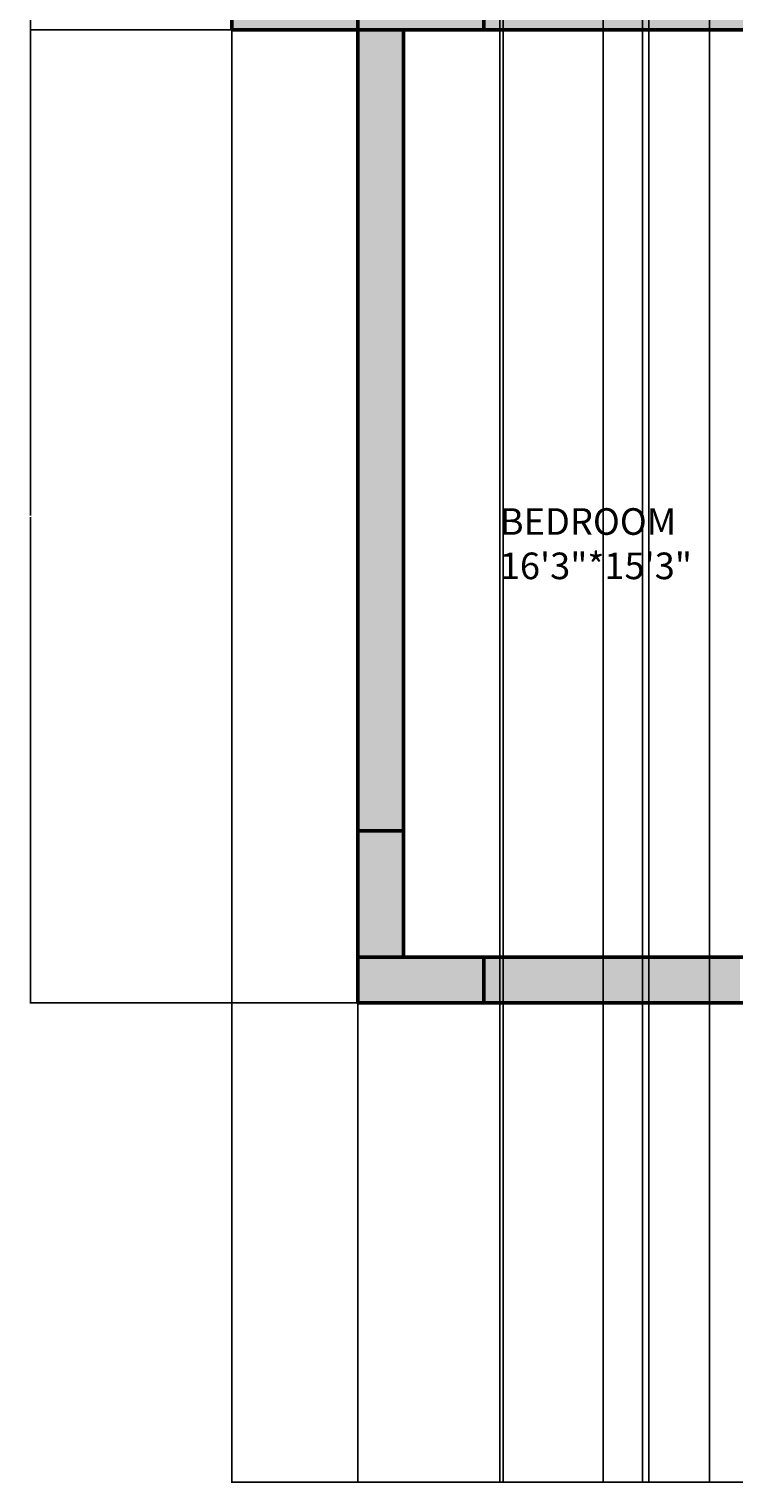
# Model space of a CAD drawing. Units: inches. Extents: x 2494 to 2908, y 1051 to 1885.
# Tile 1 of 7: x 2494 to 2634, y 1051 to 1338. Entities that reach past the tile are written whole.
import ezdxf

# ---------------------------------------------------------------- set-up
doc = ezdxf.new("R2010")
doc.units = ezdxf.units.IN
for name, color, linetype, lineweight in [('A-ANNO-DIMS', 2, 'Continuous', 18), ('A-AREA-IDEN', 130, 'Continuous', 18), ('A-COLS-PATT', 200, 'Continuous', 13), ('A-WALL-PATT', 140, 'Continuous', 13), ('COLUMN', 200, 'Continuous', 50), ('WALL', 140, 'Continuous', 50)]:
    doc.layers.add(name, color=color, linetype=linetype, lineweight=lineweight)
doc.styles.get("Standard").update_dxf_attribs({"font": 'arial.ttf'})
doc.dimstyles.get("Standard").update_dxf_attribs({"dimtxt": 0.18, "dimasz": 0.18, "dimexe": 0.18, "dimexo": 0.0625, "dimgap": 0.09, "dimtad": 0, "dimtih": 1, "dimtoh": 1, "dimdec": 4, "dimzin": 0, "dimdsep": 46, "dimtxsty": 'Standard', "dimcen": 0.09, "dimadec": 0, "dimazin": 0, "dimtfac": 1, "dimtdec": 4, "dimtofl": 0, "dimtmove": 0, "dimatfit": 3, "dimfxl": 1, "dimtolj": 1, "dimtzin": 0, "dimarcsym": 0})

# ---------------------------------------------------------------- blocks, each defined once
blk = doc.blocks.new('*D25')
at = {"layer": 'A-ANNO-DIMS', "color": 0, "lineweight": -2, "transparency": 16777216}
for p, q in [((2534.4, 1338.09), (2534.4, 1051.41)), ((2868.25, 1146.09), (2868.25, 1051.41)), ((2534.58, 1051.59), (2700.86, 1051.59)), ((2868.07, 1051.59), (2701.79, 1051.59))]:
    blk.add_line(p, q, dxfattribs=at)
at = {"layer": 'A-ANNO-DIMS', "color": 0, "lineweight": 100, "transparency": 16777216}
for points in [[(2534.58, 1051.62), (2534.58, 1051.56), (2534.4, 1051.59)], [(2868.07, 1051.62), (2868.07, 1051.56), (2868.25, 1051.59)]]:
    blk.add_solid(points, dxfattribs=at)
at = {"layer": 'Defpoints', "color": 0, "lineweight": 100, "transparency": 16777216}
for p in [(2534.4, 1338.16), (2868.25, 1146.16), (2868.25, 1051.59)]:
    blk.add_point(p, dxfattribs=at)
at = {"layer": 'A-ANNO-DIMS', "color": 0, "transparency": 16777216, "insert": (2701.33, 1051.59), "char_height": 0.18, "attachment_point": 5}
blk.add_mtext('\\A1;333.85', dxfattribs=at)
blk = doc.blocks.new('*D28')
at = {"layer": 'A-ANNO-DIMS', "color": 0, "lineweight": -2, "transparency": 16777216}
for p, q in [((2534.34, 1456.66), (2494.47, 1456.66)), ((2494.65, 1456.48), (2494.65, 1397.59)), ((2494.65, 1338.34), (2494.65, 1397.22)), ((2534.34, 1338.16), (2494.47, 1338.16))]:
    blk.add_line(p, q, dxfattribs=at)
at = {"layer": 'A-ANNO-DIMS', "color": 0, "lineweight": 100, "transparency": 16777216}
for points in [[(2494.62, 1456.48), (2494.68, 1456.48), (2494.65, 1456.66)], [(2494.62, 1338.34), (2494.68, 1338.34), (2494.65, 1338.16)]]:
    blk.add_solid(points, dxfattribs=at)
at = {"layer": 'Defpoints', "color": 0, "lineweight": 100, "transparency": 16777216}
for p in [(2494.65, 1456.66), (2534.4, 1456.66), (2534.4, 1338.16)]:
    blk.add_point(p, dxfattribs=at)
at = {"layer": 'A-ANNO-DIMS', "color": 0, "transparency": 16777216, "insert": (2494.65, 1397.41), "char_height": 0.18, "attachment_point": 5}
blk.add_mtext('\\A1;118.5', dxfattribs=at)
blk = doc.blocks.new('*D29')
at = {"layer": 'A-ANNO-DIMS', "color": 0, "lineweight": -2, "transparency": 16777216}
for p, q in [((2559.19, 1338.16), (2494.47, 1338.16)), ((2494.65, 1337.98), (2494.65, 1242.34)), ((2494.65, 1146.34), (2494.65, 1241.97)), ((2559.19, 1146.16), (2494.47, 1146.16))]:
    blk.add_line(p, q, dxfattribs=at)
at = {"layer": 'A-ANNO-DIMS', "color": 0, "lineweight": 100, "transparency": 16777216}
for points in [[(2494.62, 1337.98), (2494.68, 1337.98), (2494.65, 1338.16)], [(2494.62, 1146.34), (2494.68, 1146.34), (2494.65, 1146.16)]]:
    blk.add_solid(points, dxfattribs=at)
at = {"layer": 'Defpoints', "color": 0, "lineweight": 100, "transparency": 16777216}
for p in [(2494.65, 1338.16), (2559.25, 1338.16), (2559.25, 1146.16)]:
    blk.add_point(p, dxfattribs=at)
at = {"layer": 'A-ANNO-DIMS', "color": 0, "transparency": 16777216, "insert": (2494.65, 1242.16), "char_height": 0.18, "attachment_point": 5}
blk.add_mtext('\\A1;192', dxfattribs=at)
blk = doc.blocks.new('*D40')
at = {"layer": 'A-ANNO-DIMS', "color": 0, "lineweight": -2, "transparency": 16777216}
for p, q in [((2615.49, 1606.59), (2615.49, 1051.41)), ((2655.49, 1606.59), (2655.49, 1051.41)), ((2615.67, 1051.59), (2635.27, 1051.59)), ((2655.31, 1051.59), (2635.71, 1051.59))]:
    blk.add_line(p, q, dxfattribs=at)
at = {"layer": 'A-ANNO-DIMS', "color": 0, "lineweight": 100, "transparency": 16777216}
for points in [[(2615.67, 1051.62), (2615.67, 1051.56), (2615.49, 1051.59)], [(2655.31, 1051.62), (2655.31, 1051.56), (2655.49, 1051.59)]]:
    blk.add_solid(points, dxfattribs=at)
at = {"layer": 'Defpoints', "color": 0, "lineweight": 100, "transparency": 16777216}
for p in [(2615.49, 1606.66), (2655.49, 1606.66), (2655.49, 1051.59)]:
    blk.add_point(p, dxfattribs=at)
at = {"layer": 'A-ANNO-DIMS', "color": 0, "transparency": 16777216, "insert": (2635.49, 1051.59), "char_height": 0.18, "attachment_point": 5}
blk.add_mtext('\\A1;40', dxfattribs=at)
blk = doc.blocks.new('*D49')
at = {"layer": 'A-ANNO-DIMS', "color": 0, "lineweight": -2, "transparency": 16777216}
for p, q in [((2587.26, 1358.2), (2587.26, 1051.41)), ((2649.88, 1357.95), (2649.88, 1051.41)), ((2587.44, 1051.59), (2618.17, 1051.59)), ((2649.7, 1051.59), (2618.96, 1051.59))]:
    blk.add_line(p, q, dxfattribs=at)
at = {"layer": 'A-ANNO-DIMS', "color": 0, "lineweight": 100, "transparency": 16777216}
for points in [[(2587.44, 1051.62), (2587.44, 1051.56), (2587.26, 1051.59)], [(2649.7, 1051.62), (2649.7, 1051.56), (2649.88, 1051.59)]]:
    blk.add_solid(points, dxfattribs=at)
at = {"layer": 'Defpoints', "color": 0, "lineweight": 100, "transparency": 16777216}
for p in [(2587.26, 1358.26), (2649.88, 1358.01), (2649.88, 1051.59)]:
    blk.add_point(p, dxfattribs=at)
at = {"layer": 'A-ANNO-DIMS', "color": 0, "transparency": 16777216, "insert": (2618.57, 1051.59), "char_height": 0.18, "attachment_point": 5}
blk.add_mtext('\\A1;62.62', dxfattribs=at)
blk = doc.blocks.new('*D51')
at = {"layer": 'A-ANNO-DIMS', "color": 0, "lineweight": -2, "transparency": 16777216}
for p, q in [((2587.26, 1358.2), (2587.26, 1051.41)), ((2559.25, 1347.09), (2559.25, 1051.41)), ((2559.43, 1051.59), (2572.88, 1051.59)), ((2587.08, 1051.59), (2573.63, 1051.59))]:
    blk.add_line(p, q, dxfattribs=at)
at = {"layer": 'A-ANNO-DIMS', "color": 0, "lineweight": 100, "transparency": 16777216}
for points in [[(2559.43, 1051.62), (2559.43, 1051.56), (2559.25, 1051.59)], [(2587.08, 1051.62), (2587.08, 1051.56), (2587.26, 1051.59)]]:
    blk.add_solid(points, dxfattribs=at)
at = {"layer": 'Defpoints', "color": 0, "lineweight": 100, "transparency": 16777216}
for p in [(2587.26, 1358.26), (2559.25, 1347.16), (2559.25, 1051.59)]:
    blk.add_point(p, dxfattribs=at)
at = {"layer": 'A-ANNO-DIMS', "color": 0, "transparency": 16777216, "insert": (2573.26, 1051.59), "char_height": 0.18, "attachment_point": 5}
blk.add_mtext('\\A1;28.01', dxfattribs=at)
blk = doc.blocks.new('*D60')
at = {"layer": 'A-ANNO-DIMS', "color": 0, "lineweight": -2, "transparency": 16777216}
for p, q in [((2587.96, 1514.09), (2587.96, 1051.41)), ((2607.71, 1514.09), (2607.71, 1051.41)), ((2588.14, 1051.59), (2597.45, 1051.59)), ((2607.53, 1051.59), (2598.22, 1051.59))]:
    blk.add_line(p, q, dxfattribs=at)
at = {"layer": 'A-ANNO-DIMS', "color": 0, "lineweight": 100, "transparency": 16777216}
for points in [[(2588.14, 1051.62), (2588.14, 1051.56), (2587.96, 1051.59)], [(2607.53, 1051.62), (2607.53, 1051.56), (2607.71, 1051.59)]]:
    blk.add_solid(points, dxfattribs=at)
at = {"layer": 'Defpoints', "color": 0, "lineweight": 100, "transparency": 16777216}
for p in [(2587.96, 1514.15), (2607.71, 1514.15), (2607.71, 1051.59)]:
    blk.add_point(p, dxfattribs=at)
at = {"layer": 'A-ANNO-DIMS', "color": 0, "transparency": 16777216, "insert": (2597.83, 1051.59), "char_height": 0.18, "attachment_point": 5}
blk.add_mtext('\\A1;19.76', dxfattribs=at)
blk = doc.blocks.new('*D62')
at = {"layer": 'A-ANNO-DIMS', "color": 0, "lineweight": -2, "transparency": 16777216}
for p, q in [((2616.72, 1527.95), (2616.72, 1051.41)), ((2628.68, 1527.95), (2628.68, 1051.41)), ((2616.9, 1051.59), (2622.25, 1051.59)), ((2628.5, 1051.59), (2623.16, 1051.59))]:
    blk.add_line(p, q, dxfattribs=at)
at = {"layer": 'A-ANNO-DIMS', "color": 0, "lineweight": 100, "transparency": 16777216}
for points in [[(2616.9, 1051.62), (2616.9, 1051.56), (2616.72, 1051.59)], [(2628.5, 1051.62), (2628.5, 1051.56), (2628.68, 1051.59)]]:
    blk.add_solid(points, dxfattribs=at)
at = {"layer": 'Defpoints', "color": 0, "lineweight": 100, "transparency": 16777216}
for p in [(2616.72, 1528.01), (2628.68, 1528.01), (2628.68, 1051.59)]:
    blk.add_point(p, dxfattribs=at)
at = {"layer": 'A-ANNO-DIMS', "color": 0, "transparency": 16777216, "insert": (2622.7, 1051.59), "char_height": 0.18, "attachment_point": 5}
blk.add_mtext('\\A1;11.963', dxfattribs=at)

msp = doc.modelspace()

# ---------------------------------------------------------------- hatches: boundary and pattern name
at = {"layer": 'A-COLS-PATT'}
h = msp.add_hatch(color=256, dxfattribs=at)
h.dxf.hatch_style = 1
h.paths.add_polyline_path([(2584.1612, 1845.1561), (2559.2517, 1845.1561), (2559.2517, 1836.1561), (2584.1612, 1836.1561)])
h.paths.add_polyline_path([(2720.7462, 1845.1561), (2695.8368, 1845.1561), (2695.8368, 1836.1561), (2720.7462, 1836.1561)])
h.paths.add_polyline_path([(2868.2517, 1845.1561), (2843.3423, 1845.1561), (2843.3423, 1836.1561), (2868.2517, 1836.1561)])
h.paths.add_polyline_path([(2568.2517, 1728.1561), (2559.2517, 1728.1561), (2559.2517, 1703.2467), (2568.2517, 1703.2467)])
h.paths.add_polyline_path([(2568.2517, 1564.0885), (2559.2517, 1564.0885), (2559.2517, 1539.1791), (2568.2517, 1539.1791)])
h.paths.add_polyline_path([(2868.2517, 1554.4528), (2859.2517, 1554.4528), (2859.2517, 1529.5434), (2868.2517, 1529.5434)])
h.paths.add_polyline_path([(2806.0841, 1611.1561), (2781.1746, 1611.1561), (2781.1746, 1602.1561), (2806.0841, 1602.1561)])
h.paths.add_polyline_path([(2868.0971, 1611.1561), (2843.1877, 1611.1561), (2843.1877, 1602.1561), (2868.0971, 1602.1561)])
h.paths.add_polyline_path([(2584.1612, 1347.1561), (2559.2517, 1347.1561), (2559.2517, 1338.1561), (2584.1612, 1338.1561)])
h.paths.add_polyline_path([(2868.2517, 1347.1561), (2843.3423, 1347.1561), (2843.3423, 1338.1561), (2868.2517, 1338.1561)])
h.paths.add_polyline_path([(2568.2517, 1180.0656), (2559.2517, 1180.0656), (2559.2517, 1155.1561), (2568.2517, 1155.1561)])
h.paths.add_polyline_path([(2584.1612, 1155.1561), (2559.2517, 1155.1561), (2559.2517, 1146.1561), (2584.1612, 1146.1561)])
h.paths.add_polyline_path([(2868.2517, 1155.1561), (2843.3423, 1155.1561), (2843.3423, 1146.1561), (2868.2517, 1146.1561)])
h.paths.add_polyline_path([(2868.2517, 1180.0656), (2859.2517, 1180.0656), (2859.2517, 1155.1561), (2868.2517, 1155.1561)])
at = {"layer": 'A-WALL-PATT'}
h = msp.add_hatch(color=256, dxfattribs=at)
h.dxf.hatch_style = 1
h.paths.add_polyline_path([(2868.2517, 1836.1561), (2859.2517, 1836.1561), (2859.2517, 1611.1561), (2868.2517, 1611.1561)])
h.paths.add_polyline_path([(2715.2517, 1611.1561), (2655.4916, 1611.1561), (2655.4916, 1606.6561), (2715.2517, 1606.6561)])
h.paths.add_polyline_path([(2781.1746, 1611.1561), (2776.9029, 1611.1561), (2715.2517, 1611.1561), (2715.2517, 1606.6561), (2715.2517, 1602.1561), (2781.1746, 1602.1561)])
h.paths.add_polyline_path([(2868.0971, 1602.1561), (2859.2517, 1602.1561), (2859.2517, 1554.4528), (2868.0971, 1554.4528)])
h.paths.add_polyline_path([(2868.2517, 1529.5434), (2859.2517, 1529.5434), (2859.2517, 1347.1561), (2868.2517, 1347.1561)])
h.paths.add_polyline_path([(2868.2517, 1338.1561), (2859.2517, 1338.1561), (2859.2517, 1243.6561), (2868.2517, 1243.6561)])
h.paths.add_polyline_path([(2568.2517, 1338.1561), (2559.2517, 1338.1561), (2559.2517, 1180.0656), (2568.2517, 1180.0656)])
h.paths.add_polyline_path([(2735.7191, 1155.1561), (2697.838, 1155.1561), (2697.838, 1146.1561), (2735.7191, 1146.1561), (2735.7191, 1151.0155)])
h = msp.add_hatch(color=256, dxfattribs=at)
h.dxf.hatch_style = 1
h.paths.add_polyline_path([(2805.2517, 1547.9123), (2796.2517, 1547.9123), (2796.2517, 1530.1561), (2859.2517, 1530.1561), (2859.2517, 1539.1561), (2805.2517, 1539.1561)])
h.paths.add_polyline_path([(2568.2517, 1606.6561), (2615.4916, 1606.6561), (2615.4916, 1611.1561), (2559.2517, 1611.1561), (2559.2517, 1564.0885), (2568.2517, 1564.0885)])
h.paths.add_polyline_path([(2568.2517, 1539.1791), (2559.2517, 1539.1791), (2559.2517, 1456.6561), (2534.4016, 1456.6561), (2534.4016, 1338.1561), (2559.2517, 1338.1561), (2559.2517, 1342.6561), (2543.4016, 1342.6561), (2543.4016, 1452.1561), (2559.2517, 1452.1561), (2568.2517, 1452.1561), (2674.7517, 1452.1561), (2674.7517, 1456.6561), (2568.2517, 1456.6561)])
h.paths.add_polyline_path([(2684.6403, 1347.1561), (2674.7517, 1347.1561), (2584.1612, 1347.1561), (2584.1612, 1338.1561), (2684.6403, 1338.1561), (2684.6403, 1341.1561)])
h.paths.add_polyline_path([(2843.3423, 1347.1561), (2832.3482, 1347.1561), (2832.3482, 1338.1485), (2843.3423, 1338.1485)])
h.paths.add_polyline_path([(2634.6908, 1155.1561), (2584.1612, 1155.1561), (2584.1612, 1146.1561), (2634.6908, 1146.1561)])
h.paths.add_polyline_path([(2783.7833, 1155.1561), (2772.2517, 1155.1561), (2772.2517, 1146.1561), (2783.7833, 1146.1561)])
h.paths.add_polyline_path([(2843.3423, 1155.1561), (2819.0012, 1155.1561), (2811.9091, 1155.1561), (2811.9091, 1146.1561), (2843.3423, 1146.1561)])
h.paths.add_polyline_path([(2868.2517, 1243.6561), (2859.2517, 1243.6561), (2859.2517, 1239.1561), (2859.2517, 1180.0656), (2868.2517, 1180.0656)])

# ---------------------------------------------------------------- linework, layer by layer
at = {"layer": 'COLUMN'}
for points in [[(2559.2517, 1347.1561), (2584.1612, 1347.1561), (2584.1612, 1338.1561), (2559.2517, 1338.1561)], [(2568.2517, 1180.0656), (2568.2517, 1155.1561), (2559.2517, 1155.1561), (2559.2517, 1180.0656)], [(2559.2517, 1155.1561), (2584.1612, 1155.1561), (2584.1612, 1146.1561), (2559.2517, 1146.1561)]]:
    msp.add_lwpolyline(points, close=True, dxfattribs=at)
at = {"layer": 'WALL'}
for p, q in [((2534.4016, 1338.1561), (2534.4016, 1456.6561)), ((2559.2517, 1347.1561), (2559.2517, 1146.1561)), ((2568.2517, 1338.1561), (2534.4016, 1338.1561)), ((2568.2517, 1338.1561), (2568.2517, 1155.1561)), ((2686.3903, 1338.1561), (2568.2517, 1338.1561)), ((2568.2517, 1155.1561), (2735.7191, 1155.1561)), ((2559.2517, 1146.1561), (2736.9268, 1146.1561))]:
    msp.add_line(p, q, dxfattribs=at)
msp.add_lwpolyline([(2559.2517, 1180.0656), (2568.2517, 1180.0656), (2568.2517, 1338.1561), (2559.2517, 1338.1561)], close=True, dxfattribs=at)

# ---------------------------------------------------------------- texts
at = {"layer": 'A-AREA-IDEN', "insert": (2587.2795, 1243.7548), "char_height": 5.248177, "attachment_point": 1}
msp.add_mtext_dynamic_manual_height_columns('BEDROOM\\P16\'3"*15\'3"', width=250.978097, gutter_width=26.2409, heights=[0], dxfattribs=at)

# ---------------------------------------------------------------- dimensions: what is measured, and where the dimension line sits
at = {"layer": 'A-ANNO-DIMS'}
for base, p1, p2, override, picture, middle in [((2655.4916, 1051.5937), (2615.4916, 1606.6561), (2655.4916, 1606.6561), {"dimdec": 0, "dimlfac": 1, "dimrnd": 0, "dimzin": 0, "dimdsep": 46, "dimlunit": 2}, '*D40', (2635.4916, 1051.5937)), ((2628.6843, 1051.5937), (2616.7213, 1528.0102), (2628.6843, 1528.0102), {"dimdec": 3, "dimlfac": 1, "dimrnd": 0, "dimzin": 0, "dimdsep": 46, "dimlunit": 2}, '*D62', (2622.7028, 1051.5937)), ((2607.7136, 1051.5937), (2587.9553, 1514.1514), (2607.7136, 1514.1514), {"dimdec": 2, "dimlfac": 1, "dimrnd": 0, "dimzin": 0, "dimdsep": 46, "dimlunit": 2}, '*D60', (2597.8345, 1051.5937)), ((2559.2517, 1051.5937), (2587.2592, 1358.2585), (2559.2517, 1347.1561), {"dimdec": 2, "dimlfac": 1, "dimrnd": 0, "dimzin": 0, "dimdsep": 46, "dimlunit": 2}, '*D51', (2573.2554, 1051.5937)), ((2649.877, 1051.5937), (2587.2592, 1358.2585), (2649.877, 1358.0085), {"dimdec": 2, "dimlfac": 1, "dimrnd": 0, "dimzin": 0, "dimdsep": 46, "dimlunit": 2}, '*D49', (2618.5681, 1051.5937)), ((2868.2517, 1051.5937), (2534.4016, 1338.1561), (2868.2517, 1146.1561), {"dimdec": 2, "dimlfac": 1, "dimrnd": 0, "dimzin": 0, "dimdsep": 46, "dimlunit": 2}, '*D25', (2701.3267, 1051.5937))]:
    dim = msp.add_linear_dim(base=base, p1=p1, p2=p2, dimstyle='Standard', override=override, dxfattribs=at)
    dim.commit()
    dim.dimension.update_dxf_attribs({"geometry": picture, "text_midpoint": middle})
for base, p1, p2, override, picture, middle in [((2494.6516, 1456.6561), (2534.4016, 1338.1561), (2534.4016, 1456.6561), {"dimdec": 1, "dimlfac": 1, "dimrnd": 0, "dimzin": 0, "dimdsep": 46, "dimlunit": 2}, '*D28', (2494.6516, 1397.4061)), ((2494.6516, 1338.1561), (2559.2517, 1146.1561), (2559.2517, 1338.1561), {"dimdec": 0, "dimlfac": 1, "dimrnd": 0, "dimzin": 0, "dimdsep": 46, "dimlunit": 2}, '*D29', (2494.6516, 1242.1561))]:
    dim = msp.add_linear_dim(base=base, p1=p1, p2=p2, angle=90, dimstyle='Standard', override=override, dxfattribs=at)
    dim.commit()
    dim.dimension.update_dxf_attribs({"geometry": picture, "text_midpoint": middle})

doc.saveas('drawing.dxf')
